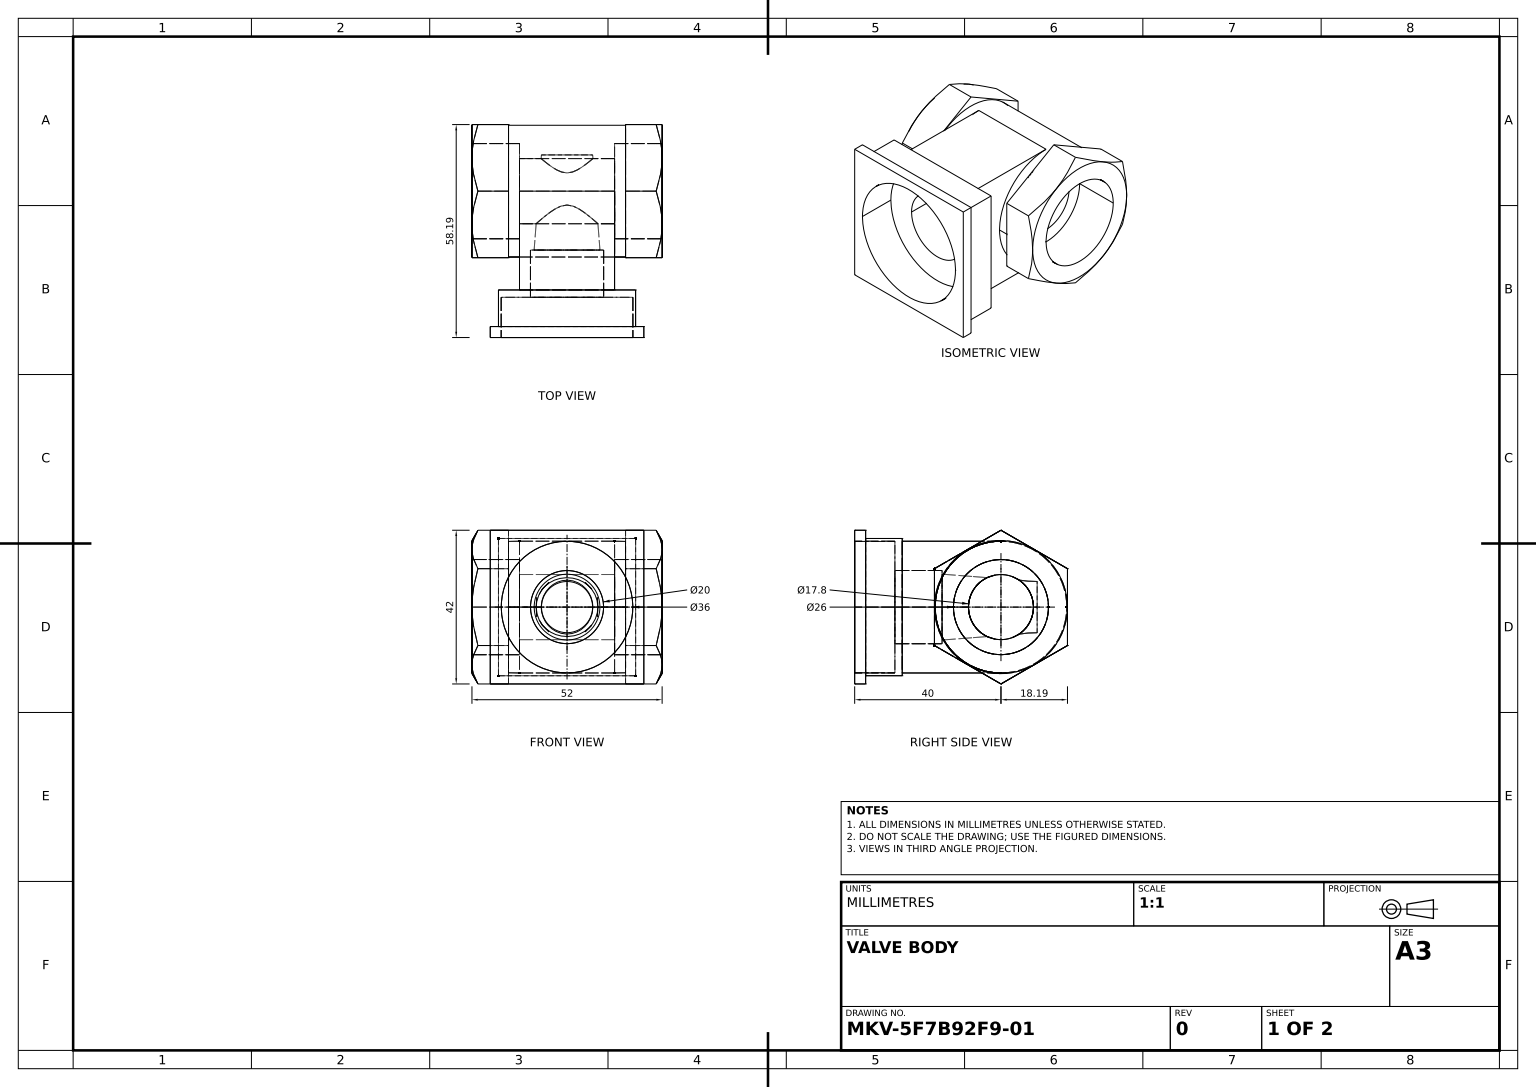
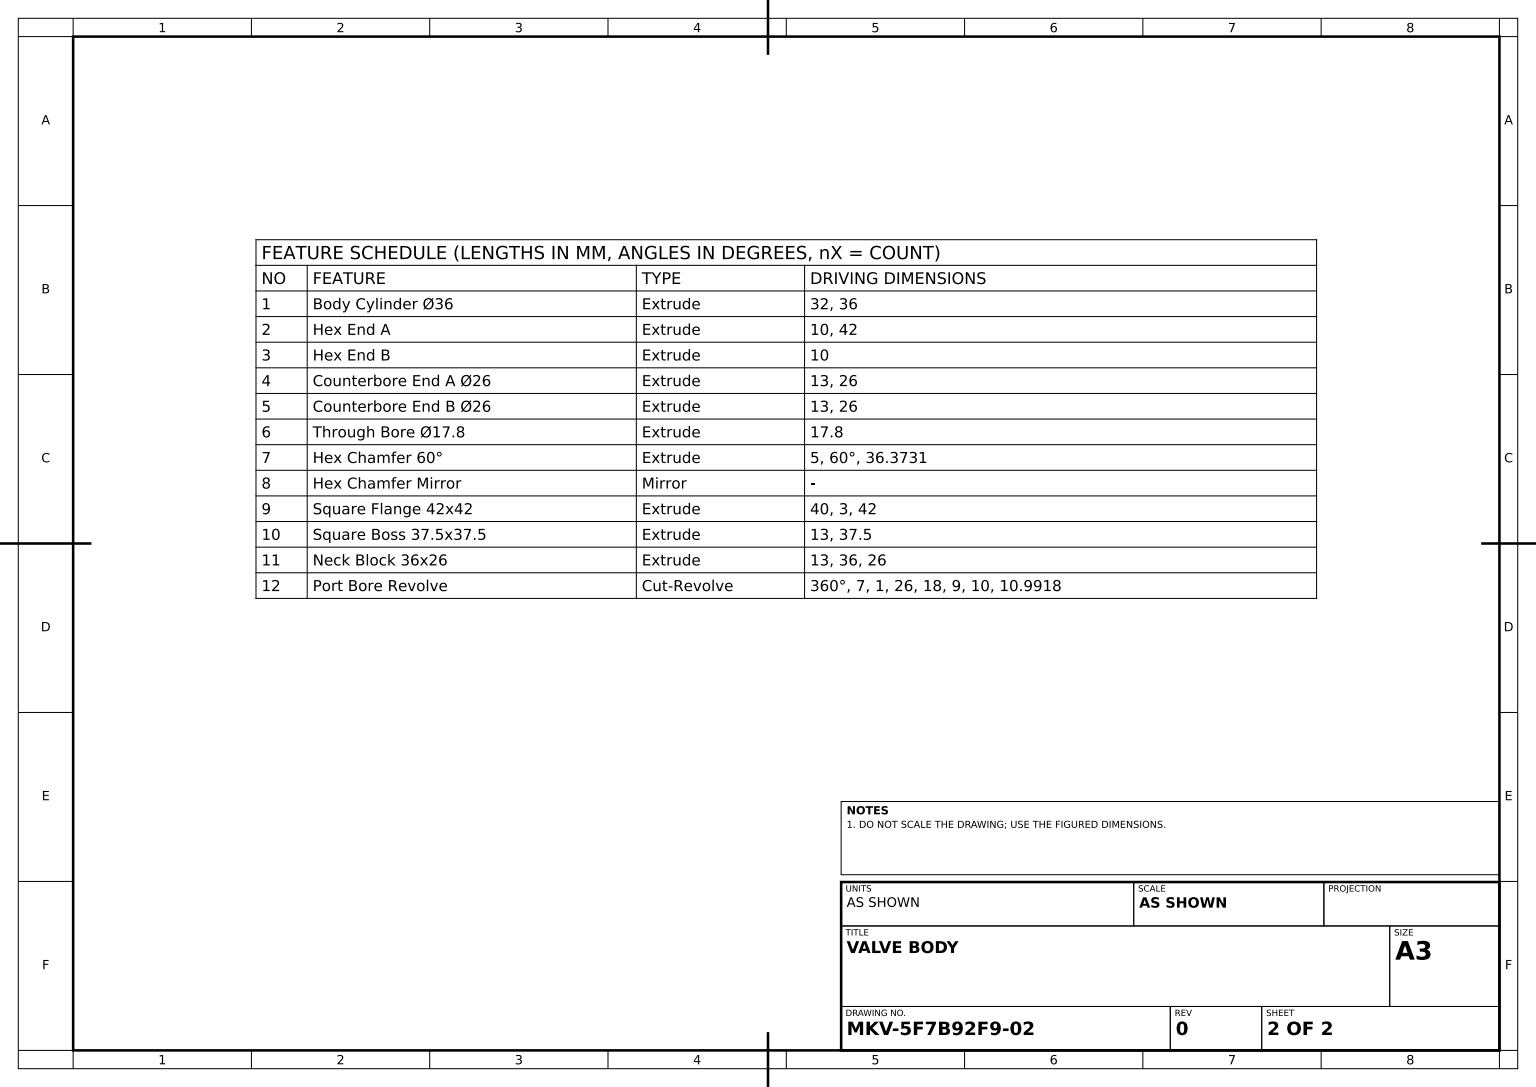
from build123d import *

# Parameters (mm, degrees)
BODY_PROFILE_36_R                  = 18
BODY_CYLINDER_36_DEPTH             = 16
HEX_END_A_DEPTH                    = 10
HEX_END_B_DEPTH                    = 10
COUNTERBORE_PROFILE_END_A_26_R     = 13
COUNTERBORE_END_A_26_DEPTH         = 13
COUNTERBORE_START                  = -13
COUNTERBORE_PROFILE_END_B_26_R     = 13
COUNTERBORE_END_B_26_DEPTH         = 13
THROUGH_BORE_PROFILE_17_8_R        = 8.9
THROUGH_BORE_17_8_DEPTH            = 48.882669099
HEX_CHAMFER_PROFILE_OUTSIDE_W      = 70.914
HEX_CHAMFER_PROFILE_OUTSIDE_H      = 76.54
HEX_CHAMFER_PROFILE_OUTSIDE_R      = 18.186533479
HEX_CHAMFER_60_DEPTH               = 5
HEX_CHAMFER_60_DRAFT               = -60
HEX_CHAMFER_MIRROR_COPY_1_SKETCH_W = 70.914
HEX_CHAMFER_MIRROR_COPY_1_SKETCH_H = 76.54
HEX_CHAMFER_MIRROR_COPY_1_SKETCH_R = 18.186533479
HEX_CHAMFER_MIRROR_COPY_1_DEPTH    = 5
HEX_CHAMFER_MIRROR_COPY_1_DRAFT    = -60
FLANGE_PROFILE_42X42_W             = 42
FLANGE_PROFILE_42X42_H             = 42
SQUARE_FLANGE_42X42_DEPTH          = 3
SQUARE_BOSS_PROFILE_37_5X37_5_W    = 37.5
SQUARE_BOSS_PROFILE_37_5X37_5_H    = 37.5
SQUARE_BOSS_37_5X37_5_DEPTH        = 13
NECK_BLOCK_36X26_REACH             = 69.102
NECK_BLOCK_36X26_END_RADIUS        = 18
NECK_BLOCK_PROFILE_36X26_W         = 26
NECK_BLOCK_PROFILE_36X26_H         = 36


with BuildPart() as part:
    # Body Profile Ø36 → Body Cylinder Ø36 (new, symmetric)
    with BuildSketch(Plane(origin=(0, 0, 0), x_dir=(0, 0, -1), z_dir=(1, 0, 0))):
        Circle(BODY_PROFILE_36_R)
    extrude(amount=BODY_CYLINDER_36_DEPTH, both=True)

    # Hex Profile End A 42 → Hex End A (add)
    with BuildSketch(Plane(origin=(16, 0, 0), x_dir=(0, 0, -1), z_dir=(1, 0, 0))):
        Polygon((0, 21), (-18.186533479, 10.5), (-18.186533479, -10.5), (0, -21), (18.186533479, -10.5), (18.186533479, 10.5), align=None)
    extrude(amount=HEX_END_A_DEPTH)

    # Hex Profile End B → Hex End B (add)
    with BuildSketch(Plane.ZY.offset(16)):
        Polygon((18.186533479, 10.5), (0, 21), (-18.186533479, 10.5), (-18.186533479, -10.5), (0, -21), (18.186533479, -10.5), align=None)
    extrude(amount=HEX_END_B_DEPTH)

    # Counterbore Profile End A Ø26 → Counterbore End A Ø26 (cut)
    with BuildSketch(Plane(origin=(26, 0, 0), x_dir=(0, 0, -1), z_dir=(1, 0, 0))):
        Circle(COUNTERBORE_PROFILE_END_A_26_R)
    extrude(amount=-COUNTERBORE_END_A_26_DEPTH, mode=Mode.SUBTRACT)

    # Counterbore Profile End B Ø26 → Counterbore End B Ø26 (cut)
    with BuildSketch(Plane.ZY.offset(26).offset(COUNTERBORE_START)):
        with Locations(Location((0, 0, 0), (0, 0, 180))):
            Circle(COUNTERBORE_PROFILE_END_B_26_R)
    extrude(amount=COUNTERBORE_END_B_26_DEPTH, mode=Mode.SUBTRACT)

    # Through Bore Profile Ø17.8 → Through Bore Ø17.8 (cut, through all)
    with BuildSketch(Plane.ZY.offset(13)):
        Circle(THROUGH_BORE_PROFILE_17_8_R)
    extrude(amount=-THROUGH_BORE_17_8_DEPTH, mode=Mode.SUBTRACT)


with BuildPart() as hex_chamfer_60_tool:
    # Hex Chamfer Profile outside → Hex Chamfer 60° (with draft: the straight prism first)
    with BuildSketch(Plane.ZY.offset(26)):
        Rectangle(HEX_CHAMFER_PROFILE_OUTSIDE_W, HEX_CHAMFER_PROFILE_OUTSIDE_H)
        Circle(HEX_CHAMFER_PROFILE_OUTSIDE_R, mode=Mode.SUBTRACT)
    extrude(amount=-HEX_CHAMFER_60_DEPTH)
    # Hex Chamfer 60°: the draft: its side faces are tilted about the plane it starts from
    hex_chamfer_60_sides = [hex_chamfer_60_tool.faces().sort_by_distance(p)[0] for p in [
        (-23.5, -38.27, 0),
        (-23.5, 0, 35.457),
        (-23.5, 38.27, 0),
        (-23.5, 0, -35.457),
        (-23.5, 0, -18.186533479),
    ]]
    draft(hex_chamfer_60_sides, Plane.ZY.offset(26), HEX_CHAMFER_60_DRAFT)


with BuildPart() as part_1:
    add(part.part)

    # Hex Chamfer 60°: cut by hex_chamfer_60_tool
    add(hex_chamfer_60_tool.part, mode=Mode.SUBTRACT)


with BuildPart() as hex_chamfer_mirror_copy_1_tool:
    # Hex Chamfer Mirror copy 1 sketch → Hex Chamfer Mirror copy 1 (with draft: the straight prism first)
    with BuildSketch(Plane(origin=(26, 0, 0), x_dir=(0, 0, 1), z_dir=(1, 0, 0))):
        Rectangle(HEX_CHAMFER_MIRROR_COPY_1_SKETCH_W, HEX_CHAMFER_MIRROR_COPY_1_SKETCH_H)
        Circle(HEX_CHAMFER_MIRROR_COPY_1_SKETCH_R, mode=Mode.SUBTRACT)
    extrude(amount=-HEX_CHAMFER_MIRROR_COPY_1_DEPTH)
    # Hex Chamfer Mirror copy 1: the draft: its side faces are tilted about the plane it starts from
    hex_chamfer_mirror_copy_1_sides = [hex_chamfer_mirror_copy_1_tool.faces().sort_by_distance(p)[0] for p in [
        (23.5, -38.27, 0),
        (23.5, 0, 35.457),
        (23.5, 38.27, 0),
        (23.5, 0, -35.457),
        (23.5, 0, -18.186533479),
    ]]
    draft(hex_chamfer_mirror_copy_1_sides, Plane(origin=(26, 0, 0), x_dir=(0, 0, 1), z_dir=(1, 0, 0)), HEX_CHAMFER_MIRROR_COPY_1_DRAFT)


with BuildPart() as part_2:
    add(part_1.part)

    # Hex Chamfer Mirror copy 1: cut by hex_chamfer_mirror_copy_1_tool
    add(hex_chamfer_mirror_copy_1_tool.part, mode=Mode.SUBTRACT)



with BuildPart() as body_2:
    # Flange Profile 42x42 → Square Flange 42x42 (new body)
    with BuildSketch(Plane.XY.offset(40)):
        Rectangle(FLANGE_PROFILE_42X42_W, FLANGE_PROFILE_42X42_H)
    extrude(amount=-SQUARE_FLANGE_42X42_DEPTH)

    # Square Boss Profile 37.5x37.5 → Square Boss 37.5x37.5 (add)
    with BuildSketch(Plane.XY.offset(40)):
        Rectangle(SQUARE_BOSS_PROFILE_37_5X37_5_W, SQUARE_BOSS_PROFILE_37_5X37_5_H)
    extrude(amount=-SQUARE_BOSS_37_5X37_5_DEPTH)


with BuildPart() as part_3:
    add(part_2.part)

    add(body_2.part)  # Neck Block 36x26 merges body 2
    # Neck Block 36x26: up to this cylinder (the profile starts outside it)
    neck_block_36x26_end = Plane(origin=(0, 0, 0), z_dir=(-1, 0, 0)) * Cylinder(NECK_BLOCK_36X26_END_RADIUS, 175.204, mode=Mode.PRIVATE)
    # Neck Block Profile 36x26 → Neck Block 36x26 (add, up to the surface)
    with BuildSketch(Plane.XY.offset(40), mode=Mode.PRIVATE) as neck_block_36x26_sk1:
        Rectangle(NECK_BLOCK_PROFILE_36X26_W, NECK_BLOCK_PROFILE_36X26_H)
    neck_block_36x26_tool1 = extrude(neck_block_36x26_sk1.sketch, amount=-NECK_BLOCK_36X26_REACH, mode=Mode.PRIVATE) - neck_block_36x26_end
    add(neck_block_36x26_tool1.solids().sort_by_distance((0, 0, 40))[0])

    # Port Bore Profile → Port Bore Revolve (revolve, cut)
    with BuildSketch(Plane(origin=(0, 0, 0), x_dir=(1, 0, 0), z_dir=(0, 1, 0))):
        Polygon((0, -40), (0, 9.9), (7, 9.9), (9, -16.1), (10, -16.1), (10, -29.008166862), (18, -29.008166862), (18, -40), align=None)
    revolve(axis=Axis((0, 0, 40), (0, 0, -1)), mode=Mode.SUBTRACT)


solid = part_3.part
